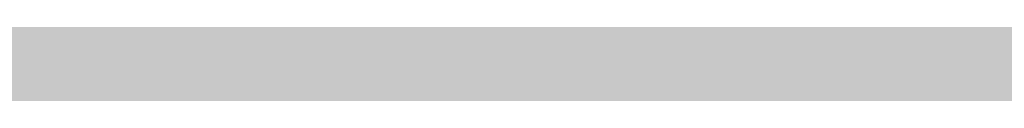
# Model space of a CAD drawing. Units: inches. Extents: x 2083 to 3317, y 1141 to 2115.
# Tile 128 of 256: x 3119.674 to 3123.979, y 1263.355 to 1263.613. Entities that reach past the tile are written whole.
import ezdxf

# ---------------------------------------------------------------- set-up
doc = ezdxf.new("R2010")
doc.units = ezdxf.units.IN
doc.layers.add('A-ANNO-DIMS', color=2, linetype='Continuous', lineweight=18)
doc.layers.add('A-WALL-PATT', color=251, linetype='Continuous', lineweight=13, true_color=0x636466)
doc.styles.get("Standard").update_dxf_attribs({"font": 'arial.ttf'})
doc.dimstyles.new('ISO-25', dxfattribs={"dimtxt": 12, "dimasz": 12, "dimexe": 1.25, "dimexo": 0.625, "dimtad": 1, "dimlunit": 3, "dimtxsty": 'Standard', "dimcen": 2.5, "dimadec": 0, "dimazin": 0, "dimtfac": 1, "dimtmove": 0, "dimatfit": 3, "dimfxl": 1, "dimarcsym": 0})

# ---------------------------------------------------------------- blocks, each defined once
blk = doc.blocks.new('*D26')
at = {"layer": 'A-ANNO-DIMS', "color": 0, "lineweight": -2, "transparency": 16777216}
for p, q in [((3088.9858, 1274.9151), (3088.9858, 1270.952)), ((3111.24, 1274.9151), (3111.24, 1270.952)), ((3076.9858, 1272.202), (2840.2624, 1272.202)), ((3111.24, 1272.202), (3088.9858, 1272.202)), ((3123.24, 1272.202), (3135.24, 1272.202))]:
    blk.add_line(p, q, dxfattribs=at)
at = {"layer": 'A-ANNO-DIMS', "color": 0, "transparency": 16777216}
for points in [[(3076.9858, 1274.202), (3076.9858, 1270.202), (3088.9858, 1272.202)], [(3123.24, 1274.202), (3123.24, 1270.202), (3111.24, 1272.202)]]:
    blk.add_solid(points, dxfattribs=at)
at = {"layer": 'Defpoints', "color": 0, "transparency": 16777216}
for p in [(3088.9858, 1275.5401), (3111.24, 1275.5401), (3088.9858, 1272.202)]:
    blk.add_point(p, dxfattribs=at)
at = {"layer": 'A-ANNO-DIMS', "color": 0, "transparency": 16777216, "insert": (2952.6241, 1279.0316), "char_height": 12, "attachment_point": 5}
blk.add_mtext('NIGHTSTAND 1\'-10 1/2" TYP.', dxfattribs=at)
blk = doc.blocks.new('*D27')
at = {"layer": 'A-ANNO-DIMS', "color": 0, "lineweight": -2, "transparency": 16777216}
for p, q in [((3114.5782, 1309.7943), (3114.5782, 1321.7943)), ((3111.865, 1297.7943), (3115.8282, 1297.7943)), ((3114.5782, 1297.7943), (3114.5782, 1275.5401)), ((3111.865, 1275.5401), (3115.8282, 1275.5401)), ((3114.5782, 1263.5401), (3114.5782, 1140.9886))]:
    blk.add_line(p, q, dxfattribs=at)
at = {"layer": 'A-ANNO-DIMS', "color": 0, "transparency": 16777216}
for points in [[(3112.5782, 1309.7943), (3116.5782, 1309.7943), (3114.5782, 1297.7943)], [(3112.5782, 1263.5401), (3116.5782, 1263.5401), (3114.5782, 1275.5401)]]:
    blk.add_solid(points, dxfattribs=at)
at = {"layer": 'Defpoints', "color": 0, "transparency": 16777216}
for p in [(3111.24, 1297.7943), (3111.24, 1275.5401), (3114.5782, 1275.5401)]:
    blk.add_point(p, dxfattribs=at)
at = {"layer": 'A-ANNO-DIMS', "color": 0, "transparency": 16777216, "insert": (3107.7485, 1196.2643), "char_height": 12, "attachment_point": 5, "rotation": 90}
blk.add_mtext('1\'-10 1/2" TYP.', dxfattribs=at)

msp = doc.modelspace()

# ---------------------------------------------------------------- hatches: boundary and pattern name
at = {"layer": 'A-WALL-PATT'}
h = msp.add_hatch(color=256, dxfattribs=at)
h.dxf.hatch_style = 1
h.paths.add_polyline_path([(3126.9598, 2020.7614), (2748.9598, 2020.7614), (2604.9598, 2020.7614), (2226.9598, 2020.7614), (2226.9598, 1702.7614), (2466.9598, 1702.7614), (2466.9598, 1582.7614), (2418.9598, 1582.7614), (2418.9598, 1477.7614), (2226.9598, 1477.7614), (2226.9598, 1263.2614), (2544.9598, 1263.2614), (2544.9598, 1411.7614), (2604.9598, 1411.7614), (2685.9598, 1411.7614), (2685.9598, 1420.7614), (2604.9598, 1420.7614), (2604.9598, 1573.7614), (2604.9598, 1702.7614), (2604.9598, 2011.7614), (2748.9598, 2011.7614), (2748.9598, 1702.7614), (2862.9598, 1702.7614), (2862.9598, 1621.7614), (2871.9598, 1621.7614), (2871.9598, 1702.7614), (2883.9598, 1702.7614), (2883.9598, 1706.9395, -0.026459), (2883.9598, 1711.7614), (2757.9598, 1711.7614), (2757.9598, 1807.7614), (2787.9598, 1807.7614), (2787.9598, 1812.2614), (2757.9598, 1812.2614), (2757.9598, 2011.7614), (2877.9598, 2011.7614), (2877.9598, 1812.2614), (2847.9598, 1812.2614), (2847.9598, 1807.7614), (2889.8357, 1807.7614), (2889.8357, 1812.2614), (2882.4598, 1812.2614), (2882.4598, 2011.7614), (3117.9598, 2011.7614), (3117.9598, 1812.2614), (2937.8357, 1812.2614), (2937.8357, 1807.7614), (2995.7098, 1807.7614), (2995.7098, 1796.1177), (3000.2098, 1796.1177), (3000.2098, 1807.7614), (3117.9598, 1807.7614), (3117.9598, 1711.7614), (3000.2098, 1711.7614), (3000.2098, 1760.1177), (2998.5727, 1760.1177, -0.020711), (2995.7098, 1760.1177), (2995.7098, 1711.7614), (2931.9598, 1711.7614), (2931.9598, 1702.7614), (3126.9598, 1702.7614)])
h.paths.add_polyline_path([(2471.4598, 2011.7614), (2471.4598, 1810.0114), (2462.7169, 1810.0114), (2462.7169, 1805.5114), (2505.9598, 1805.5114), (2505.9598, 1810.0114), (2475.9598, 1810.0114), (2475.9598, 2011.7614), (2595.9598, 2011.7614), (2595.9598, 1810.0114), (2565.9598, 1810.0114), (2565.9598, 1805.5114), (2595.9598, 1805.5114), (2595.9598, 1711.7614), (2235.9598, 1711.7614), (2235.9598, 1805.5114), (2353.7098, 1805.5114), (2353.7098, 1796.0542), (2358.2098, 1796.0542), (2358.2098, 1805.5114), (2414.7169, 1805.5114), (2414.7169, 1810.0114), (2235.9598, 1810.0114), (2235.9598, 2011.7614)], flags=16)
h.paths.add_polyline_path([(2270.2047, 1994.61), (2270.2047, 1970.61), (2246.2047, 1970.61), (2246.2047, 1994.61)], flags=0)
edge = h.paths.add_edge_path(flags=0)
edge.add_ellipse((2332.0274, 1899.7982), major_axis=(-3.043, 3.043), ratio=0.168252, start_angle=-161.3322, end_angle=-156.3071, ccw=False)
edge.add_ellipse((2333.082, 1898.7435), major_axis=(-1.0546, 1.0546), ratio=0.453532, start_angle=-123.371, end_angle=-94.1591)
edge = h.paths.add_edge_path(flags=0)
edge.add_ellipse((2332.0274, 1968.8763), major_axis=(3.043, 3.043), ratio=0.168252, start_angle=18.6678, end_angle=23.6929)
edge.add_spline(control_points=[(2332.9256, 1970.6911), (2332.2268, 1970.3361), (2330.8937, 1969.6589), (2328.4131, 1970.9321), (2327.2039, 1967.7487), (2324.7096, 1969.9556), (2322.5328, 1967.0124), (2320.0128, 1971.2958), (2317.6803, 1968.1578), (2316.0405, 1967.102), (2315.4269, 1966.8096)], knot_values=[0, 0, 0, 0, 2.267059, 4.324559, 6.685584, 8.878641, 11.121502, 14.300359, 17.755284, 19.732645, 19.732645, 19.732645, 19.732645], degree=3, periodic=0)
edge.add_ellipse((2332.0274, 1968.8763), major_axis=(3.043, 3.043), ratio=0.168252, start_angle=18.6678, end_angle=23.6929, ccw=False)
edge.add_ellipse((2333.082, 1969.9309), major_axis=(1.0546, 1.0546), ratio=0.453532, start_angle=56.629, end_angle=85.8409, ccw=False)
edge = h.paths.add_edge_path(flags=0)
edge.add_spline(control_points=[(2296.4283, 1967.9879), (2293.6278, 1965.3363), (2287.7036, 1959.7271), (2299.7439, 1949.9957), (2294.5326, 1935.6685), (2290.5732, 1920.6035), (2293.3941, 1909.9737), (2296.1854, 1904.9665)], knot_values=[0.099185, 0.099185, 0.099185, 0.099185, 0.345301, 0.619822, 0.982653, 1.386093, 1.810555, 1.810555, 1.810555, 1.810555], degree=3, periodic=0)
edge.add_spline(control_points=[(2296.1854, 1904.9665), (2297.3836, 1902.6193), (2298.001, 1901.9493), (2298.553, 1901.4682)], knot_values=[0.006246, 0.006246, 0.006246, 0.006246, 0.055476, 0.055476, 0.055476, 0.055476], degree=3, periodic=0)
edge.add_spline(control_points=[(2298.553, 1901.4682), (2297.2586, 1900.9232), (2295.2253, 1900.2321), (2293.0602, 1900.6142), (2292.1014, 1900.7884), (2292.0896, 1900.7906)], knot_values=[0.312835, 0.312835, 0.312835, 0.312835, 0.40178, 0.474987, 0.475903, 0.475903, 0.475903, 0.475903], degree=3, periodic=0)
edge.add_arc((2292.7936, 1904.6641), 3.937, 215.4209, 259.6982, ccw=False)
edge.add_spline(control_points=[(2289.5853, 1902.3823), (2289.4767, 1902.5351), (2289.3685, 1902.688), (2289.2609, 1902.8412)], knot_values=[0.102872, 0.102872, 0.102872, 0.102872, 0.116896, 0.116896, 0.116896, 0.116896], degree=3, periodic=0)
edge.add_spline(control_points=[(2289.2609, 1902.8412), (2288.6866, 1902.5502), (2287.64, 1902.0199), (2285.8813, 1901.874), (2283.853, 1901.5044), (2281.72, 1899.7105), (2278.467, 1899.4929), (2276.1571, 1901.8832), (2272.259, 1899.8041), (2267.7776, 1901.8432), (2262.2439, 1900.184), (2257.4149, 1901.7821), (2254.3184, 1900.7261), (2253.1783, 1900.3373)], knot_values=[0, 0, 0, 0, 1.907977, 3.477176, 5.261074, 7.972851, 11.680248, 13.717921, 16.939592, 22.789562, 27.502503, 33.595215, 37.145618, 37.145618, 37.145618, 37.145618], degree=3, periodic=0)
edge.add_line((2253.1783, 1900.3373), (2250.2442, 1902.8412))
edge.add_line((2250.2442, 1902.8412), (2250.2442, 1965.8333))
edge.add_line((2250.2442, 1965.8333), (2253.1783, 1968.3371))
edge.add_spline(control_points=[(2253.1783, 1968.3371), (2254.3184, 1967.9483), (2257.4149, 1966.8924), (2262.2439, 1968.4904), (2267.7776, 1966.8313), (2271.5267, 1968.5372), (2273.8759, 1967.8283), (2274.2067, 1967.7276)], knot_values=[0, 0, 0, 0, 0.09018, 0.244935, 0.364644, 0.513233, 0.537855, 0.537855, 0.537855, 0.537855], degree=3, periodic=0)
edge.add_arc((2274.3529, 1963.7933), 3.937, 72.0511, 92.1279, ccw=False)
edge.add_arc((2281.2969, 1985.23), 18.5963, 252.05113, 288.56572)
edge.add_arc((2292.3167, 1956.0289), 12.6461, 71.02679, 113.77822, ccw=False)
edge = h.paths.add_edge_path(flags=0)
edge.add_spline(control_points=[(2274.8994, 1951.8562), (2275.0662, 1951.6166), (2275.2327, 1951.3766), (2275.398, 1951.1359)], knot_values=[1.409916, 1.409916, 1.409916, 1.409916, 1.43159, 1.43159, 1.43159, 1.43159], degree=3, periodic=0)
edge.add_spline(control_points=[(2275.398, 1951.1359), (2275.7921, 1950.5619), (2276.1792, 1949.9838), (2276.5455, 1949.3971)], knot_values=[1.358238, 1.358238, 1.358238, 1.358238, 1.409916, 1.409916, 1.409916, 1.409916], degree=3, periodic=0)
edge.add_line((2276.5455, 1949.3971), (2277.4373, 1947.8622))
edge.add_spline(control_points=[(2277.4373, 1947.8622), (2276.3038, 1945.6731), (2274.6397, 1942.4269), (2274.6316, 1938.0939), (2272.7991, 1930.8515), (2274.3564, 1943.897), (2275.9477, 1947.9234), (2276.5455, 1949.3971)], knot_values=[0.005632, 0.005632, 0.005632, 0.005632, 0.186014, 0.266002, 0.357087, 0.59639, 0.739732, 0.739732, 0.739732, 0.739732], degree=3, periodic=0)
edge.add_spline(control_points=[(2276.5455, 1949.3971), (2276.1792, 1949.9838), (2275.7921, 1950.5619), (2275.398, 1951.1359)], knot_values=[1.358238, 1.358238, 1.358238, 1.358238, 1.409916, 1.409916, 1.409916, 1.409916], degree=3, periodic=0)
edge.add_spline(control_points=[(2275.398, 1951.1359), (2274.9425, 1950.0805), (2274.2078, 1948.0253), (2273.9346, 1944.8515), (2272.4685, 1937.6275), (2273.4662, 1945.6965), (2274.7006, 1951.0595), (2274.8994, 1951.8562)], knot_values=[0.104364, 0.104364, 0.104364, 0.104364, 0.189636, 0.269624, 0.36071, 0.600013, 0.644622, 0.644622, 0.644622, 0.644622], degree=3, periodic=0)
h.paths.add_polyline_path([(2269.1675, 1963.1276, -0.357527), (2268.1706, 1960.9764, -0.092561), (2268.1706, 1939.4363, -0.357527), (2269.1675, 1937.2851, -0.357527), (2267.0163, 1938.282, -0.164785), (2254.6856, 1938.282, -0.357527), (2252.5344, 1937.2851, -0.357527), (2253.5313, 1939.4363, -0.092561), (2253.5313, 1960.9764, -0.357527), (2252.5344, 1963.1276, -0.357527), (2254.6856, 1962.1307, -0.164785), (2267.0163, 1962.1307, -0.357527)], flags=0)
h.paths.add_polyline_path([(2248.8741, 1967.8018), (2248.8741, 1957.0277), (2249.4578, 1957.0277), (2249.4578, 1911.6468), (2248.8741, 1911.6468), (2248.8741, 1900.8727), (2246.5119, 1900.8727, 0.197327), (2244.1497, 1902.4569), (2244.1497, 1966.2176, 0.197327), (2246.5119, 1967.8018)], flags=0)
h.paths.add_polyline_path([(2269.1675, 1931.3893, -0.357527), (2268.1706, 1929.2381, -0.092561), (2268.1706, 1907.6981, -0.357527), (2269.1675, 1905.5469, -0.357527), (2267.0163, 1906.5438, -0.164785), (2254.6856, 1906.5438, -0.357527), (2252.5344, 1905.5469, -0.357527), (2253.5313, 1907.6981, -0.092561), (2253.5313, 1929.2381, -0.357527), (2252.5344, 1931.3893, -0.357527), (2254.6856, 1930.3925, -0.164785), (2267.0163, 1930.3925, -0.357527)], flags=0)
edge = h.paths.add_edge_path(flags=0)
edge.add_spline(control_points=[(2276.1969, 1906.7237), (2276.1681, 1909.0289), (2276.114, 1913.3719), (2270.5984, 1924.925), (2273.9052, 1919.0128), (2275.9217, 1916.2621), (2275.4746, 1912.4021), (2277.2579, 1910.3806), (2276.696, 1908.225), (2276.6462, 1906.813), (2276.6178, 1906.0084)], knot_values=[0, 0, 0, 0, 8.61026, 16.221274, 18.843057, 23.804898, 27.440828, 29.356102, 31.203478, 33.650687, 33.650687, 33.650687, 33.650687], degree=3, periodic=0)
edge.add_spline(control_points=[(2276.6178, 1906.0084), (2276.6233, 1905.6241), (2276.4977, 1904.6287), (2275.4418, 1903.8547), (2274.9373, 1903.0804), (2274.8591, 1902.8412)], knot_values=[0.156488, 0.156488, 0.156488, 0.156488, 0.184398, 0.231376, 0.250598, 0.250598, 0.250598, 0.250598], degree=3, periodic=0)
edge.add_line((2274.8591, 1902.8412), (2276.506, 1902.8412))
edge.add_spline(control_points=[(2276.506, 1902.8412), (2276.7883, 1903.0849), (2277.6651, 1904.1252), (2278.2495, 1904.3407), (2277.6539, 1908.5274), (2278.1557, 1906.2278), (2278.1005, 1905.2859), (2278.8467, 1904.069), (2277.8568, 1903.4149), (2277.8742, 1902.991), (2277.9036, 1902.8412)], knot_values=[0.059574, 0.059574, 0.059574, 0.059574, 0.080753, 0.103741, 0.16972, 0.176036, 0.207137, 0.240474, 0.262341, 0.27366, 0.27366, 0.27366, 0.27366], degree=3, periodic=0)
edge.add_line((2277.9036, 1902.8412), (2280.0298, 1902.8412))
edge.add_spline(control_points=[(2280.0298, 1902.8412), (2279.8882, 1903.0884), (2279.4993, 1903.9816), (2280.1523, 1905.9393), (2278.1036, 1909.6578), (2279.7624, 1907.1853), (2280.3279, 1904.8749), (2280.4851, 1903.4896), (2281.4633, 1903.2494), (2281.7583, 1902.9365), (2281.834, 1902.8412)], knot_values=[0.013856, 0.013856, 0.013856, 0.013856, 0.034874, 0.088867, 0.107879, 0.126738, 0.158714, 0.193757, 0.217487, 0.226722, 0.226722, 0.226722, 0.226722], degree=3, periodic=0)
edge.add_spline(control_points=[(2281.834, 1902.8412), (2281.7875, 1902.8267), (2281.647, 1902.783), (2281.3955, 1902.8595), (2281.0881, 1902.9852), (2280.7207, 1903.0609), (2280.3335, 1903.0257), (2280.1248, 1902.8989), (2280.0298, 1902.8412)], knot_values=[0, 0, 0, 0, 0.14413, 0.435517, 0.749276, 1.153046, 1.548371, 1.878348, 1.878348, 1.878348, 1.878348], degree=3, periodic=0)
edge.add_line((2280.0298, 1902.8412), (2277.9036, 1902.8412))
edge.add_spline(control_points=[(2277.9036, 1902.8412), (2277.8929, 1902.7959), (2277.8654, 1902.6796), (2277.6075, 1902.6875), (2277.2741, 1902.8007), (2276.8379, 1902.6198), (2276.5838, 1902.7893), (2276.506, 1902.8412)], knot_values=[0, 0, 0, 0, 0.127189, 0.326199, 0.628009, 1.24357, 1.515331, 1.515331, 1.515331, 1.515331], degree=3, periodic=0)
edge.add_line((2276.506, 1902.8412), (2274.8591, 1902.8412))
edge.add_spline(control_points=[(2274.8591, 1902.8412), (2274.8144, 1902.8986), (2274.7251, 1903.0134), (2274.4935, 1903.119), (2274.2443, 1902.9605), (2273.9371, 1903.1849), (2273.614, 1902.9831), (2273.4083, 1902.883), (2273.3223, 1902.8412)], knot_values=[0, 0, 0, 0, 0.21843, 0.436957, 0.687977, 0.990379, 1.398396, 1.69185, 1.69185, 1.69185, 1.69185], degree=3, periodic=0)
edge.add_spline(control_points=[(2273.3223, 1902.8412), (2273.6167, 1903.4457), (2274.274, 1904.5383), (2276.0272, 1904.5737), (2276.207, 1906.5836), (2276.1969, 1906.7237)], knot_values=[0.012227, 0.012227, 0.012227, 0.012227, 0.059472, 0.106218, 0.134458, 0.134458, 0.134458, 0.134458], degree=3, periodic=0)
h.paths.add_polyline_path([(2270.7761, 1897.7898), (2270.7761, 1873.7898), (2246.7761, 1873.7898), (2246.7761, 1897.7898)], flags=0)
h.paths.add_polyline_path([(2353.7098, 1760.0051), (2353.7098, 1760.0542), (2358.2098, 1760.0542, -0.033729)], flags=0)
h.paths.add_polyline_path([(2321.8191, 1737.5292), (2341.9953, 1737.5292, -0.414214), (2343.2033, 1736.3212), (2343.2033, 1721.0206, -0.414214), (2341.9953, 1719.8127), (2321.8191, 1719.8127, -0.414214), (2320.6112, 1721.0206), (2320.6112, 1736.3212, -0.414214)], flags=0)
h.paths.add_polyline_path([(2324.235, 1736.3212), (2339.5794, 1736.3212, -0.414214), (2341.9953, 1733.9053), (2341.9953, 1725.4497, -0.414214), (2339.5794, 1723.0338), (2333.6806, 1723.0338), (2333.8453, 1722.0455, -0.870646), (2335.4254, 1721.8259, -0.767327), (2333.9227, 1721.4232), (2331.291, 1721.4232, -0.767327), (2329.7883, 1721.8259, -0.870646), (2331.3684, 1722.0455), (2331.5331, 1723.0338), (2324.235, 1723.0338, -0.414214), (2321.8191, 1725.4497), (2321.8191, 1733.9053, -0.414214)], flags=0)
h.paths.add_polyline_path([(2570.4838, 1928.6154), (2589.6838, 1928.6154), (2590.1688, 1928.6154), (2590.1688, 1904.9934), (2570.4838, 1904.9934)], flags=0)
h.paths.add_polyline_path([(2574.4473, 1927.2638, -1), (2572.8288, 1927.2638, -1)], flags=0)
h.paths.add_polyline_path([(2573.0899, 1926.9409), (2573.925, 1927.776), (2574.1477, 1927.5533), (2573.3126, 1926.7182)], flags=0)
h.paths.add_polyline_path([(2578.7791, 1919.7296, -1), (2571.5917, 1919.7296, -1)], flags=0)
h.paths.add_polyline_path([(2578.3854, 1919.7296, -1), (2571.9854, 1919.7296, -1)], flags=0)
h.paths.add_polyline_path([(2331.5958, 1729.4762, -1), (2333.618, 1729.4762, -1)], flags=0)
h.paths.add_polyline_path([(2578.0342, 1927.2638, -1), (2576.4157, 1927.2638, -1)], flags=0)
h.paths.add_polyline_path([(2576.6889, 1927.5311), (2576.9116, 1927.7538), (2577.7467, 1926.9186), (2577.524, 1926.6959)], flags=0)
h.paths.add_polyline_path([(2578.1391, 1909.8595, -1), (2572.2317, 1909.8595, -1)], flags=0)
h.paths.add_polyline_path([(2577.7454, 1909.8595, -1), (2572.6254, 1909.8595, -1)], flags=0)
h.paths.add_polyline_path([(2583.7977, 1927.2638, -1), (2582.1792, 1927.2638, -1)], flags=0)
h.paths.add_polyline_path([(2582.7186, 1927.7538), (2583.5538, 1926.9186), (2583.3311, 1926.6959), (2582.4959, 1927.5311)], flags=0)
h.paths.add_polyline_path([(2582.4959, 1927.5311), (2582.7186, 1927.7538), (2583.5538, 1926.9186), (2583.3311, 1926.6959)], flags=0)
h.paths.add_polyline_path([(2587.7391, 1920.5296, -1), (2581.8317, 1920.5296, -1)], flags=0)
h.paths.add_polyline_path([(2587.3454, 1920.5296, -1), (2582.2254, 1920.5296, -1)], flags=0)
h.paths.add_polyline_path([(2587.3846, 1927.2638, -1), (2585.7661, 1927.2638, -1)], flags=0)
h.paths.add_polyline_path([(2586.082, 1926.9802), (2586.9172, 1927.8154), (2587.1399, 1927.5927), (2586.3047, 1926.7575)], flags=0)
h.paths.add_polyline_path([(2588.3791, 1910.6595, -1), (2581.1917, 1910.6595, -1)], flags=0)
h.paths.add_polyline_path([(2587.9854, 1910.6595, -1), (2581.5854, 1910.6595, -1)], flags=0)
h.paths.add_polyline_path([(2417.1677, 1729.4779), (2437.3439, 1729.4779, -0.414214), (2438.5519, 1728.2699), (2438.5519, 1712.9693, -0.414214), (2437.3439, 1711.7614), (2417.1677, 1711.7614, -0.414214), (2415.9598, 1712.9693), (2415.9598, 1728.2699, -0.414214)], flags=0)
h.paths.add_polyline_path([(2419.5836, 1728.2699), (2434.928, 1728.2699, -0.414214), (2437.3439, 1725.8541), (2437.3439, 1717.3984, -0.414214), (2434.928, 1714.9825), (2429.0292, 1714.9825), (2429.1939, 1713.9942, -0.870646), (2430.774, 1713.7746, -0.767327), (2429.2713, 1713.372), (2426.6396, 1713.372, -0.767327), (2425.1369, 1713.7746, -0.870646), (2426.717, 1713.9942), (2426.8817, 1714.9825), (2419.5836, 1714.9825, -0.414214), (2417.1677, 1717.3984), (2417.1677, 1725.8541, -0.414214)], flags=0)
h.paths.add_polyline_path([(2419.5836, 1728.2699), (2434.928, 1728.2699, -0.414214), (2437.3439, 1725.8541), (2437.3439, 1717.3984, -0.414214), (2434.928, 1714.9825), (2429.0292, 1714.9825), (2428.3581, 1719.009), (2427.5528, 1719.009), (2426.8817, 1714.9825), (2419.5836, 1714.9825, -0.414214), (2417.1677, 1717.3984), (2417.1677, 1725.8541, -0.414214)], flags=0)
h.paths.add_polyline_path([(2426.9444, 1721.4249, -1), (2428.9666, 1721.4249, -1)], flags=0)
h.paths.add_polyline_path([(2475.9598, 1702.7614), (2595.9598, 1702.7614), (2595.9598, 1582.7614), (2475.9598, 1582.7614)], flags=16)
h.paths.add_polyline_path([(2427.9598, 1573.7614), (2595.9598, 1573.7614), (2595.9598, 1468.7614), (2595.9598, 1420.7614), (2384.4598, 1420.7614), (2384.4598, 1468.7614), (2427.9598, 1468.7614)], flags=16)
h.paths.add_polyline_path([(2379.9598, 1468.7614), (2379.9598, 1420.7614), (2235.9598, 1420.7614), (2235.9598, 1468.7614)], flags=16)
h.paths.add_polyline_path([(2317.816, 1466.6958), (2337.9922, 1466.6958, -0.414214), (2339.2002, 1465.4878), (2339.2002, 1450.1872, -0.414214), (2337.9922, 1448.9792), (2317.816, 1448.9792, -0.414214), (2316.6081, 1450.1872), (2316.6081, 1465.4878, -0.414214)], flags=0)
h.paths.add_polyline_path([(2320.2319, 1465.4878), (2335.5763, 1465.4878, -0.414214), (2337.9922, 1463.0719), (2337.9922, 1454.6163, -0.414214), (2335.5763, 1452.2004), (2329.6775, 1452.2004), (2329.8422, 1451.212, -0.870646), (2331.4223, 1450.9925, -0.767327), (2329.9196, 1450.5898), (2327.2879, 1450.5898, -0.767327), (2325.7852, 1450.9925, -0.870646), (2327.3653, 1451.212), (2327.53, 1452.2004), (2320.2319, 1452.2004, -0.414214), (2317.816, 1454.6163), (2317.816, 1463.0719, -0.414214)], flags=0)
h.paths.add_polyline_path([(2320.2319, 1465.4878), (2335.5763, 1465.4878, -0.414214), (2337.9922, 1463.0719), (2337.9922, 1454.6163, -0.414214), (2335.5763, 1452.2004), (2329.6775, 1452.2004), (2329.0064, 1456.2269), (2328.2011, 1456.2269), (2327.53, 1452.2004), (2320.2319, 1452.2004, -0.414214), (2317.816, 1454.6163), (2317.816, 1463.0719, -0.414214)], flags=0)
h.paths.add_polyline_path([(2327.5926, 1458.6428, -1), (2329.6148, 1458.6428, -1)], flags=0)
h.paths.add_polyline_path([(2244.4117, 1433.3405), (2241.9209, 1433.3405, -0.414214), (2240.0179, 1435.2435), (2240.0179, 1440.9528, -0.414211), (2241.9209, 1442.8559), (2244.4117, 1442.8559, -1.976472)], flags=0)
h.paths.add_polyline_path([(2245.3569, 1434.3975, -0.414214), (2245.3569, 1441.7988, -2.144098)], flags=0)
h.paths.add_polyline_path([(2535.9598, 1416.2614), (2535.9598, 1272.2614), (2235.9598, 1272.2614), (2235.9598, 1416.2614)], flags=16)
h.paths.add_polyline_path([(2260.1196, 1384.2928), (2260.1196, 1362.0386), (2237.8654, 1362.0386), (2237.8654, 1384.2928)], flags=0)
edge = h.paths.add_edge_path(flags=0)
edge.add_line((2318.2518, 1362.0933), (2318.1458, 1362.001))
edge.add_ellipse((2317.4451, 1360.431), major_axis=(2.8216, 2.8216), ratio=0.168252, start_angle=18.6678, end_angle=20.9481, ccw=False)
edge.add_ellipse((2318.423, 1361.409), major_axis=(0.9779, 0.9779), ratio=0.453532, start_angle=56.629, end_angle=70.2262, ccw=False)
edge = h.paths.add_edge_path(flags=0)
edge.add_line((2319.1074, 1295.5711), (2319.015, 1295.6771))
edge.add_ellipse((2317.4451, 1296.3778), major_axis=(-2.8216, 2.8216), ratio=0.168252, start_angle=-161.3322, end_angle=-159.0519, ccw=False)
edge.add_ellipse((2318.423, 1295.3999), major_axis=(-0.9779, 0.9779), ratio=0.453532, start_angle=-123.371, end_angle=-109.7738)
edge = h.paths.add_edge_path(flags=0)
edge.add_spline(control_points=[(2284.2103, 1301.1702), (2284.5807, 1300.4447), (2284.8912, 1299.892), (2285.1596, 1299.461)], knot_values=[0.039066, 0.039066, 0.039066, 0.039066, 0.055476, 0.055476, 0.055476, 0.055476], degree=3, periodic=0)
edge.add_line((2285.1596, 1299.461), (2284.2103, 1301.1702))
edge = h.paths.add_edge_path(flags=0)
edge.add_line((2280.4125, 1297.298), (2283.37, 1297.0361))
edge.add_line((2283.37, 1297.0361), (2286.4057, 1297.9263))
edge.add_spline(control_points=[(2286.4057, 1297.9263), (2285.3055, 1297.4631), (2284.3448, 1297.1292), (2283.37, 1297.0361)], knot_values=[0.394369, 0.394369, 0.394369, 0.394369, 0.475903, 0.475903, 0.475903, 0.475903], degree=3, periodic=0)
edge.add_spline(control_points=[(2283.37, 1297.0361), (2283.2814, 1297.0277), (2282.3163, 1296.9573), (2281.3125, 1297.1345), (2280.4234, 1297.296), (2280.4125, 1297.298)], knot_values=[0.312835, 0.312835, 0.312835, 0.312835, 0.320246, 0.393453, 0.394369, 0.394369, 0.394369, 0.394369], degree=3, periodic=0)
edge = h.paths.add_edge_path(flags=0)
edge.add_line((2284.4356, 1359.6073), (2280.4463, 1355.328))
edge.add_line((2280.4463, 1355.328), (2279.58, 1351.0178))
edge.add_line((2279.58, 1351.0178), (2282.413, 1346.5804))
edge.add_spline(control_points=[(2282.413, 1346.5804), (2283.1533, 1345.5892), (2284.2529, 1344.0289), (2284.801, 1342.3872), (2284.9352, 1341.8055)], knot_values=[1.240098, 1.240098, 1.240098, 1.240098, 1.332892, 1.382712, 1.382712, 1.382712, 1.382712], degree=3, periodic=0)
edge.add_spline(control_points=[(2284.9352, 1341.8055), (2285.3191, 1340.1406), (2285.233, 1338.4092), (2284.9099, 1336.6541)], knot_values=[1.097484, 1.097484, 1.097484, 1.097484, 1.240098, 1.240098, 1.240098, 1.240098], degree=3, periodic=0)
edge.add_spline(control_points=[(2284.9099, 1336.6541), (2284.5868, 1334.899), (2284.0267, 1333.1203), (2283.4626, 1331.3606)], knot_values=[0.95487, 0.95487, 0.95487, 0.95487, 1.097484, 1.097484, 1.097484, 1.097484], degree=3, periodic=0)
edge.add_line((2283.4626, 1331.3606), (2281.8904, 1326.1534))
edge.add_line((2281.8904, 1326.1534), (2280.7563, 1321.0561))
edge.add_line((2280.7563, 1321.0561), (2280.2992, 1316.002))
edge.add_line((2280.2992, 1316.002), (2280.7159, 1310.9501))
edge.add_line((2280.7159, 1310.9501), (2282.0281, 1305.9721))
edge.add_line((2282.0281, 1305.9721), (2284.2103, 1301.1702))
edge.add_spline(control_points=[(2284.2103, 1301.1702), (2283.3407, 1302.7302), (2282.6119, 1304.3365), (2282.0281, 1305.9721)], knot_values=[0.099185, 0.099185, 0.099185, 0.099185, 0.241799, 0.241799, 0.241799, 0.241799], degree=3, periodic=0)
edge.add_spline(control_points=[(2282.0281, 1305.9721), (2281.4443, 1307.6078), (2281.0055, 1309.2728), (2280.7159, 1310.9501)], knot_values=[0.241799, 0.241799, 0.241799, 0.241799, 0.384413, 0.384413, 0.384413, 0.384413], degree=3, periodic=0)
edge.add_spline(control_points=[(2280.7159, 1310.9501), (2280.4332, 1312.5876), (2280.2894, 1314.277), (2280.2989, 1315.962), (2280.2992, 1316.002)], knot_values=[0.384413, 0.384413, 0.384413, 0.384413, 0.523647, 0.527028, 0.527028, 0.527028, 0.527028], degree=3, periodic=0)
edge.add_spline(control_points=[(2280.2992, 1316.002), (2280.3123, 1317.687), (2280.4779, 1319.3679), (2280.7563, 1321.0561)], knot_values=[0.527028, 0.527028, 0.527028, 0.527028, 0.669642, 0.669642, 0.669642, 0.669642], degree=3, periodic=0)
edge.add_spline(control_points=[(2280.7563, 1321.0561), (2281.0346, 1322.7443), (2281.4259, 1324.4396), (2281.8904, 1326.1534)], knot_values=[0.669642, 0.669642, 0.669642, 0.669642, 0.812256, 0.812256, 0.812256, 0.812256], degree=3, periodic=0)
edge.add_spline(control_points=[(2281.8904, 1326.1534), (2282.2644, 1327.5333), (2282.7879, 1329.2618), (2283.3528, 1331.0178), (2283.4626, 1331.3606)], knot_values=[0.812256, 0.812256, 0.812256, 0.812256, 0.927087, 0.95487, 0.95487, 0.95487, 0.95487], degree=3, periodic=0)
edge.add_line((2283.4626, 1331.3606), (2284.9099, 1336.6541))
edge.add_line((2284.9099, 1336.6541), (2284.9352, 1341.8055))
edge.add_line((2284.9352, 1341.8055), (2282.413, 1346.5804))
edge.add_spline(control_points=[(2282.413, 1346.5804), (2281.2751, 1348.1038), (2280.0784, 1349.5703), (2279.58, 1351.0178)], knot_values=[1.382712, 1.382712, 1.382712, 1.382712, 1.525326, 1.525326, 1.525326, 1.525326], degree=3, periodic=0)
edge.add_spline(control_points=[(2279.58, 1351.0178), (2279.4433, 1351.4147), (2279.1363, 1352.8569), (2279.7352, 1354.2904), (2280.4463, 1355.328)], knot_values=[1.525326, 1.525326, 1.525326, 1.525326, 1.564439, 1.667941, 1.667941, 1.667941, 1.667941], degree=3, periodic=0)
edge.add_spline(control_points=[(2280.4463, 1355.328), (2281.4261, 1356.7578), (2282.9308, 1358.1826), (2284.4356, 1359.6073)], knot_values=[1.667941, 1.667941, 1.667941, 1.667941, 1.810555, 1.810555, 1.810555, 1.810555], degree=3, periodic=0)
edge.add_arc((2280.6231, 1348.5182), 11.7262, 71.02679, 113.77822)
edge.add_arc((2270.4049, 1375.5952), 17.2436, 252.05113, 288.56572, ccw=False)
edge.add_arc((2263.966, 1355.7178), 3.6506, 72.0511, 92.1279)
edge.add_arc((2263.966, 1355.7178), 3.6506, 92.1279, 177.9851)
edge.add_spline(control_points=[(2260.3176, 1355.8462), (2260.2604, 1354.2207), (2260.5513, 1350.1865), (2262.9993, 1346.7663), (2264.4727, 1344.649)], knot_values=[1.43159, 1.43159, 1.43159, 1.43159, 1.564144, 1.770695, 1.770695, 1.770695, 1.770695], degree=3, periodic=0)
edge.add_line((2264.4727, 1344.649), (2264.9356, 1343.9825))
edge.add_spline(control_points=[(2263.801, 1340.2481), (2263.8432, 1340.5141), (2264.0672, 1341.7565), (2264.5127, 1343.0025), (2264.935, 1343.9811)], knot_values=[0.53657, 0.53657, 0.53657, 0.53657, 0.559349, 0.644622, 0.644622, 0.644622, 0.644622], degree=3, periodic=0)
edge.add_spline(control_points=[(2264.935, 1343.9811), (2265.1178, 1343.715), (2265.2989, 1343.4479), (2265.4768, 1343.1794)], knot_values=[1.384077, 1.384077, 1.384077, 1.384077, 1.409916, 1.409916, 1.409916, 1.409916], degree=3, periodic=0)
edge.add_spline(control_points=[(2265.4768, 1343.1794), (2265.6546, 1342.9108), (2265.8293, 1342.6408), (2265.9991, 1342.3688)], knot_values=[1.358238, 1.358238, 1.358238, 1.358238, 1.384077, 1.384077, 1.384077, 1.384077], degree=3, periodic=0)
edge.add_line((2265.9991, 1342.3688), (2266.826, 1340.9455))
edge.add_spline(control_points=[(2266.826, 1340.9455), (2268.8944, 1337.0897), (2271.3982, 1325.843), (2270.5162, 1310.5686), (2275.9194, 1301.8606), (2277.7895, 1299.1994)], knot_values=[0.116896, 0.116896, 0.116896, 0.116896, 0.472987, 1.050969, 1.313793, 1.313793, 1.313793, 1.313793], degree=3, periodic=0)
edge.add_spline(control_points=[(2277.7895, 1299.1994), (2277.8394, 1299.1285), (2277.8894, 1299.0575), (2277.9396, 1298.9866)], knot_values=[0.109884, 0.109884, 0.109884, 0.109884, 0.116896, 0.116896, 0.116896, 0.116896], degree=3, periodic=0)
edge.add_line((2277.9396, 1298.9866), (2277.7888, 1299.1991))
edge.add_spline(control_points=[(2277.7888, 1299.1991), (2277.2566, 1298.9294), (2276.2864, 1298.4379), (2275.0394, 1298.3344), (2274.3833, 1298.2389), (2274.2153, 1298.2093)], knot_values=[33.12187, 33.12187, 33.12187, 33.12187, 35.029056, 36.598255, 37.144827, 37.144827, 37.144827, 37.144827], degree=3, periodic=0)
edge.add_line((2274.2153, 1298.2093), (2273.0731, 1297.893))
edge.add_spline(control_points=[(2273.0731, 1297.893), (2272.3229, 1297.5798), (2271.0392, 1296.5105), (2269.2484, 1296.2261), (2268.4231, 1296.3747)], knot_values=[26.532584, 26.532584, 26.532584, 26.532584, 29.198919, 31.839101, 31.839101, 31.839101, 31.839101], degree=3, periodic=0)
edge.add_line((2268.4231, 1296.3747), (2263.8785, 1297.4575))
edge.add_spline(control_points=[(2263.8785, 1297.4575), (2263.5561, 1297.3594), (2261.8603, 1296.8387), (2260.2388, 1297.2824), (2258.9335, 1297.5165)], knot_values=[15.919551, 15.919551, 15.919551, 15.919551, 16.939592, 21.226067, 21.226067, 21.226067, 21.226067], degree=3, periodic=0)
edge.add_line((2258.9335, 1297.5165), (2254.0552, 1297.329))
edge.add_spline(control_points=[(2254.0552, 1297.329), (2253.7555, 1297.2958), (2252.1137, 1297.1652), (2250.4619, 1297.5442), (2249.1297, 1297.6679)], knot_values=[5.306517, 5.306517, 5.306517, 5.306517, 6.276435, 10.613034, 10.613034, 10.613034, 10.613034], degree=3, periodic=0)
edge.add_line((2249.1297, 1297.6679), (2244.3316, 1296.8778))
edge.add_line((2244.3316, 1296.8778), (2241.611, 1299.1994))
edge.add_line((2241.611, 1299.1994), (2241.611, 1357.6094))
edge.add_line((2241.611, 1357.6094), (2244.3316, 1359.9311))
edge.add_line((2244.3316, 1359.9311), (2252.7288, 1359.5427))
edge.add_spline(control_points=[(2252.7288, 1359.5427), (2252.8709, 1359.5464), (2253.3057, 1359.5482), (2253.7398, 1359.5143), (2254.0317, 1359.4824)], knot_values=[0.233291, 0.233291, 0.233291, 0.233291, 0.244935, 0.268927, 0.268927, 0.268927, 0.268927], degree=3, periodic=0)
edge.add_line((2254.0317, 1359.4824), (2259.5872, 1359.4164))
edge.add_spline(control_points=[(2259.5872, 1359.4164), (2260.6771, 1359.6285), (2262.0732, 1359.897), (2263.5237, 1359.4593), (2263.8304, 1359.366)], knot_values=[0.422516, 0.422516, 0.422516, 0.422516, 0.513233, 0.537855, 0.537855, 0.537855, 0.537855], degree=3, periodic=0)
edge.add_arc((2263.966, 1355.7178), 3.6506, 72.0511, 92.1279, ccw=False)
edge.add_arc((2270.4049, 1375.5952), 17.2436, 252.05113, 288.56572)
edge.add_arc((2280.6231, 1348.5182), 11.7262, 71.02679, 113.77822, ccw=False)
h.paths.add_polyline_path([(2240.3405, 1359.4347), (2240.3405, 1349.4444), (2240.8818, 1349.4444), (2240.8818, 1307.3645), (2240.3405, 1307.3645), (2240.3405, 1297.3741), (2238.1502, 1297.3741, 0.197327), (2235.9598, 1298.8431), (2235.9598, 1357.9657, 0.197327), (2238.1502, 1359.4347)], flags=0)
h.paths.add_polyline_path([(2259.1578, 1355.1005, -0.357527), (2258.2334, 1353.1058, -0.092561), (2258.2334, 1333.1326, -0.357527), (2259.1578, 1331.1379, -0.357527), (2257.1631, 1332.0622, -0.164785), (2245.7293, 1332.0622, -0.357527), (2243.7346, 1331.1379, -0.357527), (2244.6589, 1333.1326, -0.092561), (2244.6589, 1353.1058, -0.357527), (2243.7346, 1355.1005, -0.357527), (2245.7293, 1354.1761, -0.164785), (2257.1631, 1354.1761, -0.357527)], flags=0)
edge = h.paths.add_edge_path(flags=0)
edge.add_line((2265.9991, 1342.3688), (2266.826, 1340.9455))
edge.add_line((2266.826, 1340.9455), (2265.3076, 1337.8141))
edge.add_line((2265.3076, 1337.8141), (2264.3582, 1334.6529))
edge.add_line((2264.3582, 1334.6529), (2264.262, 1333.7997))
edge.add_spline(control_points=[(2264.262, 1333.7997), (2264.2084, 1333.1871), (2264.1621, 1332.3655), (2264.0071, 1331.4139), (2263.969, 1331.2018)], knot_values=[0.464444, 0.464444, 0.464444, 0.464444, 0.516691, 0.531608, 0.531608, 0.531608, 0.531608], degree=3, periodic=0)
edge.add_spline(control_points=[(2263.969, 1331.2018), (2263.7745, 1330.1189), (2263.4244, 1328.7908), (2263.2574, 1328.5307), (2263.234, 1328.5146)], knot_values=[0.372682, 0.372682, 0.372682, 0.372682, 0.44885, 0.464444, 0.464444, 0.464444, 0.464444], degree=3, periodic=0)
edge.add_spline(control_points=[(2263.234, 1328.5146), (2263.0964, 1328.4202), (2263.1312, 1329.3015), (2263.275, 1330.6157)], knot_values=[0.280919, 0.280919, 0.280919, 0.280919, 0.372682, 0.372682, 0.372682, 0.372682], degree=3, periodic=0)
edge.add_spline(control_points=[(2263.275, 1330.6157), (2263.4187, 1331.93), (2263.6715, 1333.6773), (2263.9699, 1335.315)], knot_values=[0.189157, 0.189157, 0.189157, 0.189157, 0.280919, 0.280919, 0.280919, 0.280919], degree=3, periodic=0)
edge.add_spline(control_points=[(2263.9699, 1335.315), (2264.1005, 1336.0322), (2264.4188, 1337.6219), (2264.7548, 1338.8644), (2264.9474, 1339.4911)], knot_values=[0.097394, 0.097394, 0.097394, 0.097394, 0.137578, 0.189157, 0.189157, 0.189157, 0.189157], degree=3, periodic=0)
edge.add_spline(control_points=[(2264.9474, 1339.4911), (2265.29, 1340.6061), (2265.6442, 1341.494), (2265.9991, 1342.3688)], knot_values=[0.005632, 0.005632, 0.005632, 0.005632, 0.097394, 0.097394, 0.097394, 0.097394], degree=3, periodic=0)
h.paths.add_polyline_path([(2259.1578, 1325.671, -0.357527), (2258.2334, 1323.6763, -0.092561), (2258.2334, 1303.7031, -0.357527), (2259.1578, 1301.7084, -0.357527), (2257.1631, 1302.6327, -0.164785), (2245.7293, 1302.6327, -0.357527), (2243.7346, 1301.7084, -0.357527), (2244.6589, 1303.7031, -0.092561), (2244.6589, 1323.6763, -0.357527), (2243.7346, 1325.671, -0.357527), (2245.7293, 1324.7466, -0.164785), (2257.1631, 1324.7466, -0.357527)], flags=0)
edge = h.paths.add_edge_path(flags=0)
edge.add_spline(control_points=[(2261.7089, 1317.3114), (2261.6795, 1317.4176), (2261.7619, 1317.3885), (2262.4907, 1316.0899), (2262.9622, 1315.3009)], knot_values=[14.955861, 14.955861, 14.955861, 14.955861, 16.221274, 18.694826, 18.694826, 18.694826, 18.694826], degree=3, periodic=0)
edge.add_spline(control_points=[(2262.9622, 1315.3009), (2262.9904, 1315.2536), (2263.7021, 1314.0674), (2264.349, 1313.1272), (2264.7301, 1312.1642)], knot_values=[18.694826, 18.694826, 18.694826, 18.694826, 18.843057, 22.433791, 22.433791, 22.433791, 22.433791], degree=3, periodic=0)
edge.add_spline(control_points=[(2264.7301, 1312.1642), (2264.8756, 1311.7964), (2265.1769, 1310.7698), (2265.1431, 1309.5593), (2265.2477, 1308.8242)], knot_values=[22.433791, 22.433791, 22.433791, 22.433791, 23.804898, 26.172756, 26.172756, 26.172756, 26.172756], degree=3, periodic=0)
edge.add_line((2265.2477, 1308.8242), (2265.8508, 1307.1719))
edge.add_spline(control_points=[(2265.8508, 1307.1719), (2266.065, 1306.8217), (2266.3844, 1306.3322), (2266.4244, 1305.7805), (2266.4204, 1305.6112)], knot_values=[28.062562, 28.062562, 28.062562, 28.062562, 29.356102, 29.911721, 29.911721, 29.911721, 29.911721], degree=3, periodic=0)
edge.add_spline(control_points=[(2266.4204, 1305.6112), (2266.4161, 1305.4326), (2266.394, 1305.25), (2266.3648, 1305.0659)], knot_values=[29.911721, 29.911721, 29.911721, 29.911721, 30.497837, 30.497837, 30.497837, 30.497837], degree=3, periodic=0)
edge.add_line((2266.3648, 1305.0659), (2266.0662, 1302.1363))
edge.add_spline(control_points=[(2266.0662, 1302.1363), (2266.0712, 1301.78), (2265.9981, 1301.2), (2265.6633, 1300.759), (2265.5089, 1300.5859)], knot_values=[0.156488, 0.156488, 0.156488, 0.156488, 0.184398, 0.203543, 0.203543, 0.203543, 0.203543], degree=3, periodic=0)
edge.add_line((2265.5089, 1300.5859), (2264.4353, 1299.1994))
edge.add_line((2264.4353, 1299.1994), (2265.9624, 1299.1994))
edge.add_line((2265.9624, 1299.1994), (2267.336, 1301.1753))
edge.add_line((2267.336, 1301.1753), (2267.3117, 1301.9862))
edge.add_spline(control_points=[(2267.3117, 1301.9862), (2267.2611, 1302.8624), (2267.1602, 1303.7371), (2267.2715, 1303.3259)], knot_values=[0.126229, 0.126229, 0.126229, 0.126229, 0.166617, 0.166617, 0.166617, 0.166617], degree=3, periodic=0)
edge.add_spline(control_points=[(2267.2715, 1303.3259), (2267.28, 1303.2943), (2267.3098, 1303.1754), (2267.3735, 1302.8836), (2267.4061, 1302.6828), (2267.4179, 1302.601)], knot_values=[0.166617, 0.166617, 0.166617, 0.166617, 0.16972, 0.176036, 0.180765, 0.180765, 0.180765, 0.180765], degree=3, periodic=0)
edge.add_spline(control_points=[(2267.7439, 1300.9875), (2267.6876, 1301.1509), (2267.4805, 1301.6567), (2267.4838, 1302.1448), (2267.4179, 1302.601)], knot_values=[0.180765, 0.180765, 0.180765, 0.180765, 0.193767, 0.220139, 0.220139, 0.220139, 0.220139], degree=3, periodic=0)
edge.add_line((2267.4179, 1302.601), (2267.7439, 1300.9875))
edge.add_spline(control_points=[(2267.7439, 1300.9875), (2267.832, 1300.7319), (2267.932, 1300.3099), (2267.5548, 1299.9745), (2267.4294, 1299.8292)], knot_values=[0.220139, 0.220139, 0.220139, 0.220139, 0.240474, 0.25489, 0.25489, 0.25489, 0.25489], degree=3, periodic=0)
edge.add_line((2267.4294, 1299.8292), (2267.2584, 1299.1994))
edge.add_line((2267.2584, 1299.1994), (2269.23, 1299.1994))
edge.add_spline(control_points=[(2269.23, 1299.1994), (2269.0987, 1299.4287), (2268.8428, 1300.0163), (2269.0116, 1300.9159), (2268.9468, 1301.6607)], knot_values=[0.013856, 0.013856, 0.013856, 0.013856, 0.034874, 0.067073, 0.067073, 0.067073, 0.067073], degree=3, periodic=0)
edge.add_line((2268.9468, 1301.6607), (2268.4316, 1303.6031))
edge.add_spline(control_points=[(2268.4316, 1303.6031), (2268.1756, 1304.1924), (2267.5962, 1305.2513), (2268.0407, 1304.6232), (2268.2514, 1304.2824)], knot_values=[0.090155, 0.090155, 0.090155, 0.090155, 0.107879, 0.120289, 0.120289, 0.120289, 0.120289], degree=3, periodic=0)
edge.add_spline(control_points=[(2268.2514, 1304.2824), (2268.3609, 1304.1053), (2269.0578, 1302.918), (2269.3827, 1301.5904), (2269.5214, 1300.7759), (2269.5752, 1300.5558)], knot_values=[0.120289, 0.120289, 0.120289, 0.120289, 0.126738, 0.158714, 0.173506, 0.173506, 0.173506, 0.173506], degree=3, periodic=0)
edge.add_line((2269.5752, 1300.5558), (2270.6858, 1299.4213))
edge.add_spline(control_points=[(2270.6858, 1299.4213), (2270.7672, 1299.3573), (2270.8379, 1299.2814), (2270.9029, 1299.1994)], knot_values=[0.21816, 0.21816, 0.21816, 0.21816, 0.226722, 0.226722, 0.226722, 0.226722], degree=3, periodic=0)
edge.add_line((2270.9372, 1299.1929), (2270.9029, 1299.1994))
edge.add_spline(control_points=[(2270.9029, 1299.1994), (2270.8598, 1299.186), (2270.7295, 1299.1455), (2270.4963, 1299.2164), (2270.2717, 1299.3083), (2270.121, 1299.348), (2270.0633, 1299.3596)], knot_values=[0.939174, 0.939174, 0.939174, 0.939174, 1.083304, 1.374691, 1.68845, 1.878348, 1.878348, 1.878348, 1.878348], degree=3, periodic=0)
edge.add_line((2270.0633, 1299.3596), (2269.23, 1299.1994))
edge.add_line((2269.23, 1299.1994), (2267.2584, 1299.1994))
edge.add_spline(control_points=[(2267.2584, 1299.1994), (2267.2484, 1299.1574), (2267.223, 1299.0497), (2266.9838, 1299.0569), (2266.8092, 1299.1162), (2266.6769, 1299.1091), (2266.6365, 1299.1048)], knot_values=[0.757665, 0.757665, 0.757665, 0.757665, 0.884854, 1.083864, 1.385675, 1.515331, 1.515331, 1.515331, 1.515331], degree=3, periodic=0)
edge.add_spline(control_points=[(2266.6365, 1299.1048), (2266.4852, 1299.0888), (2266.2358, 1299.0171), (2266.0346, 1299.1513), (2265.9624, 1299.1994)], knot_values=[0, 0, 0, 0, 0.485905, 0.757665, 0.757665, 0.757665, 0.757665], degree=3, periodic=0)
edge.add_line((2265.9624, 1299.1994), (2264.4353, 1299.1994))
edge.add_line((2264.4353, 1299.1994), (2263.8584, 1299.3671))
edge.add_spline(control_points=[(2263.8584, 1299.3671), (2263.8189, 1299.3709), (2263.7795, 1299.3857), (2263.7401, 1299.4015)], knot_values=[0.845925, 0.845925, 0.845925, 0.845925, 0.978627, 0.978627, 0.978627, 0.978627], degree=3, periodic=0)
edge.add_line((2263.7218, 1299.3964), (2263.0103, 1299.1994))
edge.add_spline(control_points=[(2263.0103, 1299.1994), (2263.2458, 1299.6829), (2263.506, 1300.1281), (2263.8735, 1300.408)], knot_values=[0.012227, 0.012227, 0.012227, 0.012227, 0.052971, 0.052971, 0.052971, 0.052971], degree=3, periodic=0)
edge.add_spline(control_points=[(2263.8735, 1300.408), (2263.9321, 1300.4527), (2264.0842, 1300.553), (2264.2552, 1300.6242), (2264.3597, 1300.6647)], knot_values=[0.052971, 0.052971, 0.052971, 0.052971, 0.059472, 0.069086, 0.069086, 0.069086, 0.069086], degree=3, periodic=0)
edge.add_line((2264.3597, 1300.6647), (2265.1419, 1301.0778))
edge.add_line((2265.1419, 1301.0778), (2265.6758, 1302.7996))
edge.add_line((2265.6758, 1302.7996), (2265.5407, 1305.7041))
edge.add_line((2265.5407, 1305.7041), (2264.8031, 1309.3277))
edge.add_line((2264.8031, 1309.3277), (2263.0405, 1314.0918))
edge.add_spline(control_points=[(2263.0405, 1314.0918), (2262.3836, 1315.6714), (2261.796, 1316.9977), (2261.7089, 1317.3114)], knot_values=[11.216896, 11.216896, 11.216896, 11.216896, 14.955861, 14.955861, 14.955861, 14.955861], degree=3, periodic=0)
h.paths.add_polyline_path([(2871.9598, 1416.2614), (2895.91, 1416.2614), (2895.91, 1420.7614), (2871.9598, 1420.7614), (2871.9598, 1501.7614), (2862.9598, 1501.7614), (2862.9598, 1420.7614), (2805.9598, 1420.7614), (2805.9598, 1411.7614), (2862.9598, 1411.7614), (2862.9598, 1263.2614), (3126.9598, 1263.2614), (3126.9598, 1411.7614), (3126.9598, 1486.7614), (2943.9598, 1486.7614), (2943.9598, 1477.7614), (2967.8603, 1477.7614), (2967.8603, 1420.7614), (2943.91, 1420.7614), (2943.91, 1416.2614), (3117.9598, 1416.2614), (3117.9598, 1420.7614), (2972.3603, 1420.7614), (2972.3603, 1477.7614), (3117.9598, 1477.7614), (3117.9598, 1420.7614), (3117.9598, 1272.2614), (2871.9598, 1272.2614)], flags=0)
h.paths.add_polyline_path([(2457.1256, 1485.9425), (2527.6027, 1485.9425), (2527.6027, 1537.6357), (2457.1256, 1537.6357)], flags=8)
h.paths.add_polyline_path([(2481.0051, 1609.9818), (2590.7658, 1609.9818), (2590.7658, 1682.0034), (2481.0051, 1682.0034)], flags=8)
h.paths.add_polyline_path([(2483.085, 1729.1268), (2553.562, 1729.1268), (2553.562, 1780.82), (2483.085, 1780.82)], flags=8)
h = msp.add_hatch(color=256, dxfattribs=at)
h.dxf.hatch_style = 1
h.paths.add_polyline_path([(3126.9598, 1486.7614), (2943.9598, 1486.7614), (2943.9598, 1477.7614), (2967.8603, 1477.7614), (2967.8603, 1420.7614), (2943.91, 1420.7614), (2943.91, 1416.2614), (3117.9598, 1416.2614), (3117.9598, 1420.7614), (2972.3603, 1420.7614), (2972.3603, 1477.7614), (3117.9598, 1477.7614), (3117.9598, 1420.7614), (3117.9598, 1272.2614), (2871.9598, 1272.2614), (2871.9598, 1416.2614), (2895.91, 1416.2614), (2895.91, 1420.7614), (2871.9598, 1420.7614), (2871.9598, 1501.7614), (2862.9598, 1501.7614), (2862.9598, 1420.7614), (2805.9598, 1420.7614), (2805.9598, 1411.7614), (2862.9598, 1411.7614), (2862.9598, 1263.2614), (3126.9598, 1263.2614), (3126.9598, 1411.7614)])

# ---------------------------------------------------------------- dimensions: what is measured, and where the dimension line sits
at = {"layer": 'A-ANNO-DIMS'}
for base, p1, p2, angle, text, picture, middle in [((3114.5782, 1275.5401), (3111.24, 1297.7943), (3111.24, 1275.5401), 270, '<> TYP.', '*D27', (3107.7485, 1196.2643)), ((3088.9858, 1272.202), (3111.24, 1275.5401), (3088.9858, 1275.5401), 180, 'NIGHTSTAND <> TYP.', '*D26', (2952.6241, 1279.0316))]:
    dim = msp.add_linear_dim(base=base, p1=p1, p2=p2, angle=angle, text=text, dimstyle='ISO-25', override={"dimdec": 1, "dimlfac": 1, "dimrnd": 0, "dimzin": 1, "dimdsep": 46, "dimlunit": 4, "dimfrac": 2}, dxfattribs=at)
    dim.commit()
    dim.dimension.update_dxf_attribs({"geometry": picture, "text_midpoint": middle})

doc.saveas('drawing.dxf')
